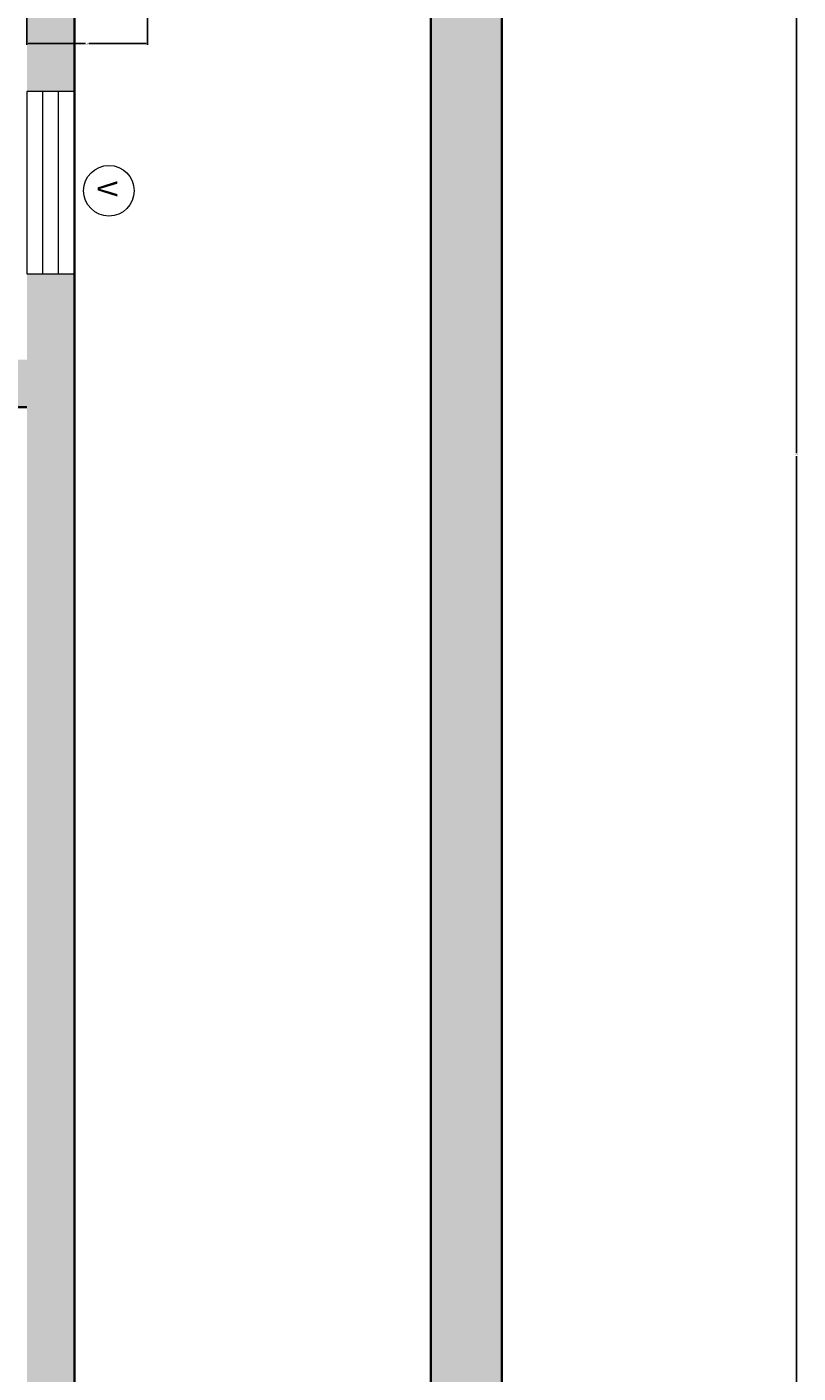
# Model space of a CAD drawing. Units: inches. Extents: x 2701 to 6846, y 811 to 2447.
# Tile 15 of 20: x 3086 to 3183, y 1130 to 1300. Entities that reach past the tile are written whole.
import ezdxf

# ---------------------------------------------------------------- set-up
doc = ezdxf.new("R2010")
doc.units = ezdxf.units.IN
for name, color, linetype, lineweight in [('A-ANNO-DIMS', 2, 'Continuous', 18), ('A-GLAZ', 4, 'Continuous', 18), ('A-WALL', 7, 'Continuous', 35), ('C-PROP', 7, 'Continuous', 35)]:
    doc.layers.add(name, color=color, linetype=linetype, lineweight=lineweight)
doc.layers.add('A-WALL-PATT', color=18, linetype='Continuous', lineweight=13, true_color=0x000000)
doc.layers.add('C-PROP-PATT', color=18, linetype='Continuous', lineweight=13, true_color=0x000000)
doc.styles.get("Standard").update_dxf_attribs({"font": 'arial.ttf'})
doc.dimstyles.get("Standard").update_dxf_attribs({"dimtxt": 0.18, "dimasz": 0.18, "dimexe": 0.18, "dimexo": 0.0625, "dimgap": 0.09, "dimtad": 0, "dimtih": 1, "dimtoh": 1, "dimdec": 4, "dimzin": 0, "dimdsep": 46, "dimtxsty": 'Standard', "dimcen": 0.09, "dimadec": 0, "dimazin": 0, "dimtfac": 1, "dimtdec": 4, "dimtofl": 0, "dimtmove": 0, "dimatfit": 3, "dimfxl": 1, "dimtolj": 1, "dimtzin": 0, "dimarcsym": 0})

# ---------------------------------------------------------------- blocks, each defined once
blk = doc.blocks.new('V')
for p, q in [((3304.15, 1279.33), (3281.15, 1279.33)), ((3304.15, 1277.33), (3281.15, 1277.33)), ((3304.15, 1275.33), (3281.15, 1275.33)), ((3281.15, 1273.33), (3304.15, 1273.33))]:
    blk.add_line(p, q)
blk.add_circle((3293.67, 1283.69), 3.19)
at = {"insert": (3292.45, 1284.76), "char_height": 2.5, "attachment_point": 1}
blk.add_mtext_dynamic_manual_height_columns('V', width=0.0153, gutter_width=12.5, heights=[0], dxfattribs=at)
blk = doc.blocks.new('V1')
for p, q in [((3281.15, 1279.33), (3281.15, 1273.33)), ((3304.15, 1273.33), (3304.15, 1279.33))]:
    blk.add_line(p, q)
blk.add_blockref('V', (0, 0))
blk = doc.blocks.new('*D34')
at = {"layer": 'A-ANNO-DIMS', "color": 0, "lineweight": -2, "transparency": 16777216}
for p, q in [((3085.97, 1305.99), (3085.97, 1297.77)), ((3101.22, 1305.99), (3101.22, 1297.77)), ((3086.15, 1297.95), (3093.38, 1297.95)), ((3101.04, 1297.95), (3093.81, 1297.95))]:
    blk.add_line(p, q, dxfattribs=at)
at = {"layer": 'A-ANNO-DIMS', "color": 0, "transparency": 16777216}
for points in [[(3086.15, 1297.98), (3086.15, 1297.92), (3085.97, 1297.95)], [(3101.04, 1297.98), (3101.04, 1297.92), (3101.22, 1297.95)]]:
    blk.add_solid(points, dxfattribs=at)
at = {"layer": 'Defpoints', "color": 0, "transparency": 16777216}
for p in [(3085.97, 1306.05), (3101.22, 1306.05), (3101.22, 1297.95)]:
    blk.add_point(p, dxfattribs=at)
at = {"layer": 'A-ANNO-DIMS', "color": 0, "transparency": 16777216, "insert": (3093.59, 1297.95), "char_height": 0.18, "attachment_point": 5}
blk.add_mtext('\\A1;15', dxfattribs=at)
blk = doc.blocks.new('*D68')
at = {"layer": 'A-ANNO-DIMS', "color": 0, "lineweight": -2, "transparency": 16777216}
for p, q in [((3092.03, 1462.05), (3183.35, 1462.05)), ((3183.17, 1461.87), (3183.17, 1246.23)), ((3183.17, 1030.23), (3183.17, 1245.87)), ((3092.03, 1030.05), (3183.35, 1030.05))]:
    blk.add_line(p, q, dxfattribs=at)
at = {"layer": 'A-ANNO-DIMS', "color": 0, "transparency": 16777216}
for points in [[(3183.14, 1461.87), (3183.2, 1461.87), (3183.17, 1462.05)], [(3183.14, 1030.23), (3183.2, 1030.23), (3183.17, 1030.05)]]:
    blk.add_solid(points, dxfattribs=at)
at = {"layer": 'Defpoints', "color": 0, "transparency": 16777216}
for p in [(3091.97, 1462.05), (3183.17, 1462.05), (3091.97, 1030.05)]:
    blk.add_point(p, dxfattribs=at)
at = {"layer": 'A-ANNO-DIMS', "color": 0, "transparency": 16777216, "insert": (3183.17, 1246.05), "char_height": 0.18, "attachment_point": 5}
blk.add_mtext('\\A1;432', dxfattribs=at)

msp = doc.modelspace()

# ---------------------------------------------------------------- hatches: boundary and pattern name
at = {"layer": 'A-WALL-PATT'}
h = msp.add_hatch(color=256, dxfattribs=at)
h.dxf.hatch_style = 1
h.paths.add_polyline_path([(3085.97, 1456.05), (3085.97, 1348.05), (3091.97, 1348.05), (3091.97, 1360.05), (3091.97, 1462.05), (2960.09, 1462.05), (2960.09, 1456.05), (2971.97, 1456.05), (2971.97, 1372.05), (2923.97, 1372.05), (2923.97, 1378.05), (2917.97, 1378.05), (2917.97, 1351.05), (2923.97, 1351.05), (2923.97, 1366.05), (2971.97, 1366.05), (2971.97, 1351.05), (2976.77, 1351.05), (2977.97, 1351.05), (2977.97, 1456.05)])
h.paths.add_polyline_path([(2779.97, 1462.05), (2779.97, 1342.05), (2785.97, 1342.05), (2785.97, 1456.05), (2917.97, 1456.05), (2917.97, 1408.05), (2922.33, 1408.05), (2923.97, 1408.05), (2923.97, 1456.05), (2937.09, 1456.05), (2937.09, 1462.05)])
h.paths.add_polyline_path([(2779.97, 1306.05), (2779.97, 1294.24), (2785.97, 1294.24), (2785.97, 1306.05), (2851.37, 1306.05, -0.025815), (2852.62, 1306.11, -0.025815), (2853.87, 1306.05), (2863.97, 1306.05), (2863.97, 1258.05), (2857.97, 1258.05), (2857.97, 1252.05), (2878.97, 1252.05), (2878.97, 1258.05), (2869.97, 1258.05), (2869.97, 1306.05), (2923.97, 1306.05), (2923.97, 1318.05), (2919.17, 1318.05), (2917.97, 1318.05), (2917.97, 1312.05), (2785.97, 1312.05), (2785.97, 1318.05), (2779.97, 1318.05)])
h.paths.add_polyline_path([(2785.97, 1252.05), (2827.97, 1252.05), (2827.97, 1256.41), (2827.97, 1258.05), (2785.97, 1258.05), (2785.97, 1271.24), (2779.97, 1271.24), (2779.97, 1174.05), (2785.97, 1174.05)])
h.paths.add_polyline_path([(2779.97, 1030.05), (2869.97, 1030.05), (2869.97, 1036.05), (2785.97, 1036.05), (2785.97, 1126.05), (2917.97, 1126.05), (2917.97, 1120.05), (2923.97, 1120.05), (2923.97, 1258.05), (2911.97, 1258.05), (2911.97, 1253.25), (2911.97, 1252.05), (2917.97, 1252.05), (2917.97, 1132.05), (2785.97, 1132.05), (2785.97, 1144.05), (2779.97, 1144.05)])
h.paths.add_polyline_path([(2935.97, 1030.05), (2935.97, 1033.05), (2935.97, 1036.05), (2923.97, 1036.05), (2923.97, 1087.05), (2919.17, 1087.05), (2917.97, 1087.05), (2917.97, 1036.05), (2893.97, 1036.05), (2893.97, 1030.05)])
h.paths.add_polyline_path([(2971.97, 1036.05), (2971.97, 1030.05), (3091.97, 1030.05), (3091.97, 1060.05), (3085.97, 1060.05), (3085.97, 1036.05)])
h.paths.add_polyline_path([(3085.97, 1084.05), (3091.97, 1084.05), (3091.97, 1096.05), (3091.97, 1268.89), (3085.97, 1268.89), (3085.97, 1258.05), (3001.97, 1258.05), (3001.97, 1270.05), (2995.97, 1270.05), (2995.97, 1252.05), (3085.97, 1252.05)])
h.paths.add_polyline_path([(3085.97, 1306.05), (3085.97, 1291.89), (3091.97, 1291.89), (3091.97, 1318.05), (3085.97, 1318.05), (3085.97, 1312.05), (2977.97, 1312.05), (2977.97, 1318.05), (2971.97, 1318.05), (2971.97, 1306.05), (2995.97, 1306.05), (2995.97, 1300.05), (3000.33, 1300.05), (3001.97, 1300.05), (3001.97, 1306.05)])
at = {"layer": 'C-PROP-PATT'}
h = msp.add_hatch(color=256, dxfattribs=at)
h.dxf.hatch_style = 1
h.paths.add_polyline_path([(3145.97, 1504.05), (2737.97, 1504.05), (2737.97, 967.05), (2746.97, 967.05), (2746.97, 1495.05), (3136.97, 1495.05), (3136.97, 865.05), (3130.97, 865.05), (3130.97, 856.05), (3145.97, 856.05)])
h.paths.add_polyline_path([(3070.97, 865.05), (2746.97, 865.05), (2746.97, 871.05), (2737.97, 871.05), (2737.97, 856.05), (3070.97, 856.05)], flags=17)

# ---------------------------------------------------------------- linework, layer by layer
at = {"layer": 'A-WALL'}
for p, q in [((3091.97, 1462.05), (3091.97, 1030.05)), ((3085.97, 1252.05), (2995.97, 1252.05))]:
    msp.add_line(p, q, dxfattribs=at)
at = {"layer": 'C-PROP'}
for p, q in [((3145.97, 1504.05), (3145.97, 856.05)), ((3136.97, 1495.05), (3136.97, 865.05))]:
    msp.add_line(p, q, dxfattribs=at)

# ---------------------------------------------------------------- block references
at = {"layer": 'A-GLAZ', "rotation": 270}
msp.add_blockref('V1', (1812.64, 4573.04), dxfattribs=at)

# ---------------------------------------------------------------- dimensions: what is measured, and where the dimension line sits
at = {"layer": 'A-ANNO-DIMS'}
dim = msp.add_linear_dim(base=(3183.17, 1462.05), p1=(3091.97, 1030.05), p2=(3091.97, 1462.05), angle=90, dimstyle='Standard', override={"dimdec": 0, "dimlfac": 1, "dimrnd": 0, "dimzin": 0, "dimdsep": 46, "dimlunit": 2}, dxfattribs=at)
dim.commit()
dim.dimension.update_dxf_attribs({"geometry": '*D68', "text_midpoint": (3183.17, 1246.05)})
dim = msp.add_linear_dim(base=(3101.22, 1297.95), p1=(3085.97, 1306.05), p2=(3101.22, 1306.05), dimstyle='Standard', override={"dimdec": 0, "dimlfac": 1, "dimrnd": 0, "dimzin": 0, "dimdsep": 46, "dimlunit": 2}, dxfattribs=at)
dim.commit()
dim.dimension.update_dxf_attribs({"geometry": '*D34', "text_midpoint": (3093.59, 1297.95)})

doc.saveas('drawing.dxf')
